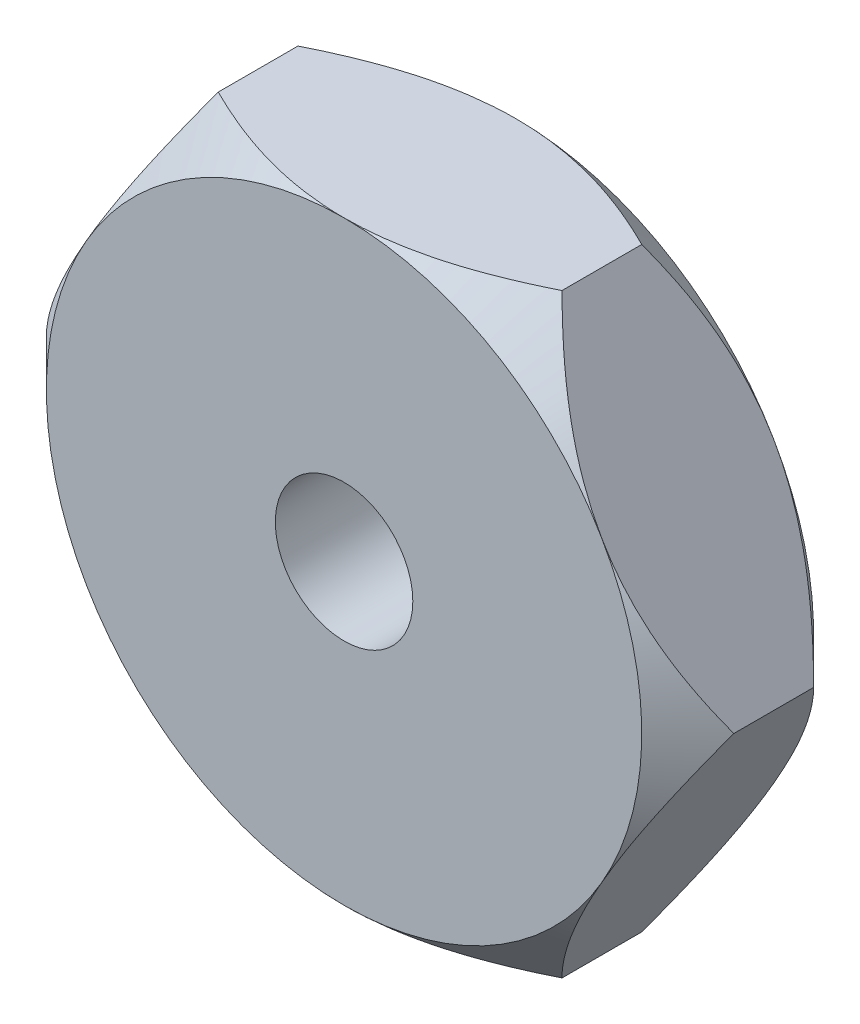
SolidWorks part; units mm, degrees
material "Plain Carbon Steel"
ref_plane "Front Plane" through (0, 0, 0) normal (0, 0, 1) x (1, 0, 0)
ref_plane "Top Plane" through (0, 0, 0) normal (0, 1, 0) x (1, 0, 0)
ref_plane "Right Plane" through (0, 0, 0) normal (1, 0, 0) x (0, 0, -1)
sketch "Hex Profile Sketch" plane through (0, 0, 0) normal (0, 0, 1) x (1, 0, 0)
  line L2 (10, 0) -> (5, 8.6603)
  line L3 (5, 8.6603) -> (-5, 8.6603)
  line L4 (-5, 8.6603) -> (-10, 0)
  line L5 (-10, 0) -> (-5, -8.6603)
  line L6 (-5, -8.6603) -> (5, -8.6603)
  line L7 (5, -8.6603) -> (10, 0)
  circle A0 centre (0, 0) radius 8.6603 construction
  dimension "D1" = 10
extrude "Hex Body" add sketch "Hex Profile Sketch" along normal mid plane 5
sketch "Bore Sketch" plane through (0, 0, 2.5) normal (0, 0, 1) x (1, 0, 0)
  circle A0 centre (0, 0) radius 2
  dimension "D1" = 4
extrude "Bore Ø4" cut sketch "Bore Sketch" against normal through all
sketch "Corner Chamfer Sketch" plane through (0, 0, 2.5) normal (0, 0, 1) x (1, 0, 0)
  line L0 (10, 0) -> (5, 8.6603) construction
  circle A0 centre (0, 0) radius 8.6603
extrude "Corner Chamfer 45deg" cut sketch "Corner Chamfer Sketch" against normal blind 5 draft 45 flip side to cut
mirror "Corner Chamfer Mirror" about plane through (0, 0, 0) normal (0, 0, 1) of "Corner Chamfer 45deg"
